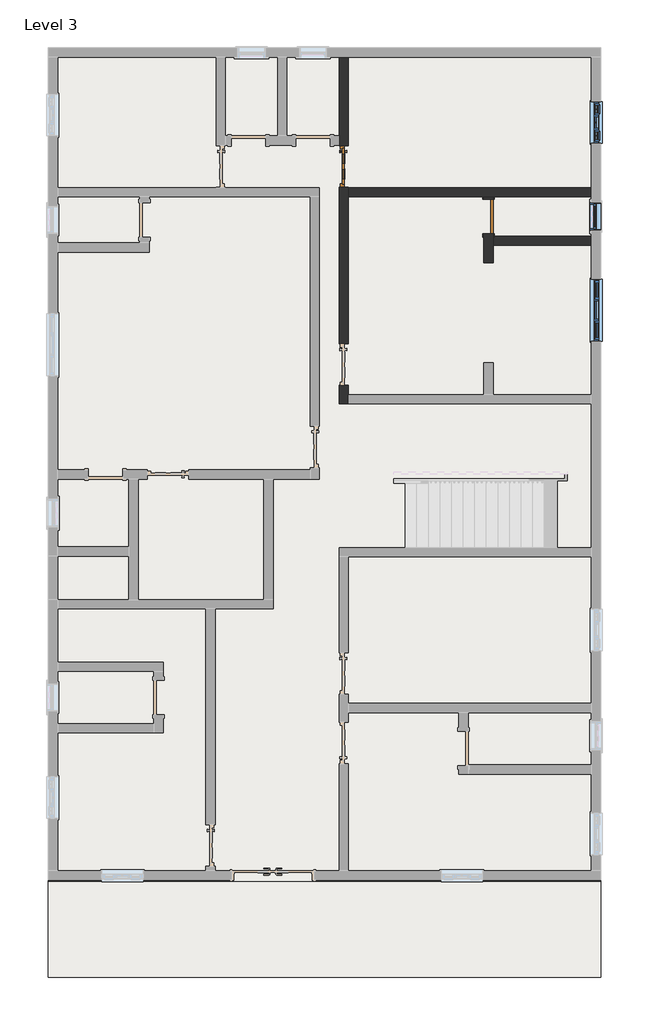
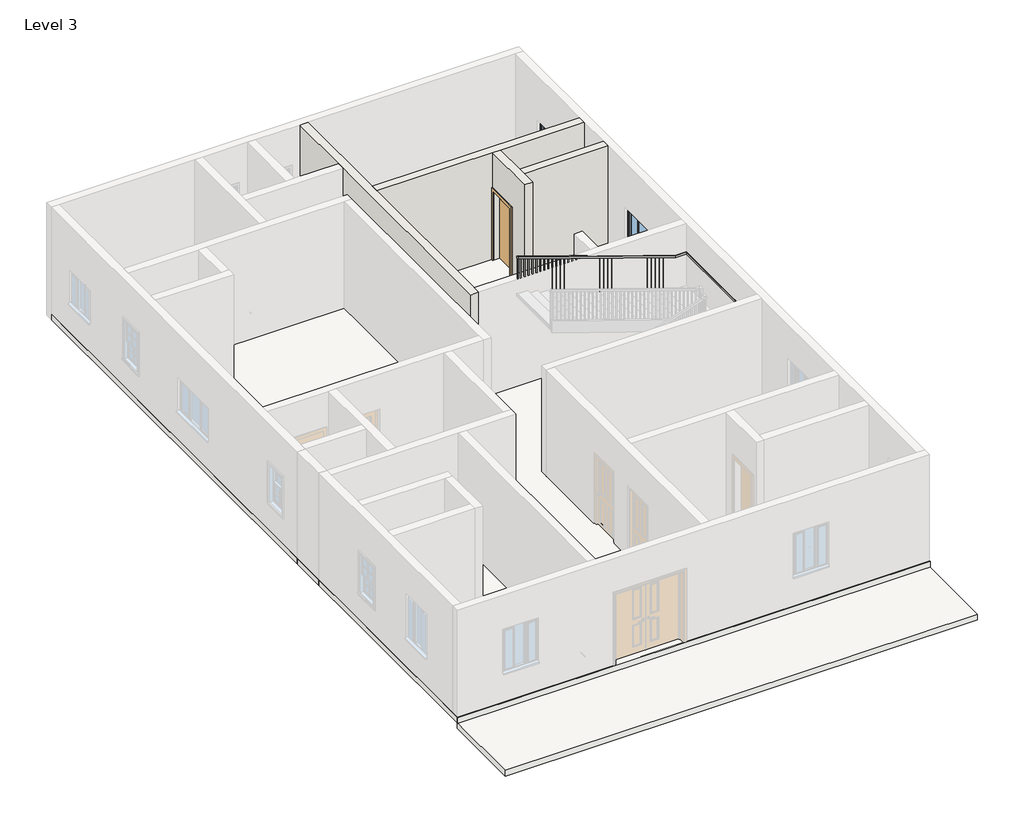
# One storey, part 2 of 3: 4 walls, 3 roofs, 3 windows, 2 doors, 1 railing, 1 slab.
"""IFC4 building model written with IfcOpenShell, lengths in millimetres."""

from ifc_helpers import new_model, si_unit, frame, origin, place, context, project, spatial, polyline, outline, extrude, faceted_brep, transform, mapped, element, save
from components import door_51b0c682, door_fadea3f2, window_679d2811, windows_tpl_plain_1360x910mm_84993ef1, windows_tpl_w_glazing_cross_bars_910x910mm_4aa0f884

model = new_model("IFC4")

# Units and contexts
model_context = context("Model", 3, world=origin())
ifc_project = project(units=[si_unit("LENGTHUNIT", "METRE", prefix="MILLI")], contexts=[model_context])

# Site, building, storey
site = spatial("IfcSite", under=ifc_project)
building = spatial("IfcBuilding", under=site)
storey = spatial("IfcBuildingStorey", under=building, Name="Level 3", Elevation=6096.0)

# Doors
placement = place(None, origin())
door_shape = door_51b0c682(model_context)
element("IfcDoor", 1, ObjectType="Doors_ExtSgl_2 : 2'x7\"", at=placement, inside=storey, context=model_context, shape_type="MappedRepresentation", body=[
    mapped(door_shape, transform((348.5548051, 6357.8803322, 6096.0), x_axis=(0.0, -1.0, 0.0), y_axis=(1.0, 0.0, 0.0), z_axis=(0.0, 0.0, 1.0))),
])
door_2_shape = door_fadea3f2(model_context)
element("IfcDoor", 2, ObjectType="Single-Flush : 30\" x 80\"", at=placement, inside=storey, context=model_context, shape_type="MappedRepresentation", body=[
    mapped(door_2_shape, transform((3523.5548051, 5259.3303322, 6096.0), x_axis=(0.0, -1.0, 0.0), y_axis=(1.0, 0.0, 0.0), z_axis=(0.0, 0.0, 1.0))),
])

# Railing
element("IfcRailing", 3, ObjectType="Handrail - Rectangular", at=placement, inside=storey, context=model_context, shape_type="SolidModel", body=[
    faceted_brep([(1449.3932247, -2014.4659014, 7096.125), (1449.3932247, -2014.4659014, 7042.4913852), (1449.3932247, -2065.2659014, 7042.4913852), (1449.3932247, -2065.2659014, 7096.125), (5246.6669505, -2014.4659014, 8382.0), (5255.0348019, -2014.4659014, 8331.2), (5255.0348019, -2065.2659014, 8331.2), (5246.6669505, -2065.2659014, 8382.0), (5771.4548051, -2014.4659014, 8382.0), (5771.4548051, -2014.4659014, 8331.2), (5822.2548051, -2065.2659014, 8331.2), (5822.2548051, -2065.2659014, 8382.0), (5771.4548051, 1135.1340986, 8382.0), (5771.4548051, 1135.1340986, 8331.2), (5822.2548051, 1185.9340986, 8331.2), (5822.2548051, 1185.9340986, 8382.0), (5499.8185322, 1135.1340986, 8382.0), (5491.4506807, 1135.1340986, 8331.2), (5491.4506807, 1185.9340986, 8331.2), (5499.8185322, 1185.9340986, 8382.0), (1449.3932247, 1135.1340986, 9753.6), (1449.3932247, 1185.9340986, 9753.6), (1449.3932247, 1185.9340986, 9699.9663852), (1449.3932247, 1135.1340986, 9699.9663852)], [[[0, 1, 2, 3]], [[1, 0, 4, 5]], [[2, 1, 5, 6]], [[3, 2, 6, 7]], [[0, 3, 7, 4]], [[5, 4, 8, 9]], [[6, 5, 9, 10]], [[7, 6, 10, 11]], [[4, 7, 11, 8]], [[9, 8, 12, 13]], [[10, 9, 13, 14]], [[11, 10, 14, 15]], [[8, 11, 15, 12]], [[13, 12, 16, 17]], [[14, 13, 17, 18]], [[15, 14, 18, 19]], [[12, 15, 19, 16]], [[20, 21, 22, 23]], [[17, 16, 20, 23]], [[18, 17, 23, 22]], [[19, 18, 22, 21]], [[16, 19, 21, 20]]]),
    extrude(outline(polyline([(9669.5618562, 1539.1798051), (9676.0127788, 1520.1298051), (8753.475, 1520.1298051), (8753.475, 1539.1798051), (9669.5618562, 1539.1798051)])), frame((0.0, 1151.0090986, 0.0), z_axis=(0.0, 1.0, 0.0), x_axis=(0.0, 0.0, 1.0)), (0.0, 0.0, 1.0), 19.05),
    extrude(outline(polyline([(9635.1569359, 1640.7798051), (9641.6078585, 1621.7298051), (8753.475, 1621.7298051), (8753.475, 1640.7798051), (9635.1569359, 1640.7798051)])), frame((0.0, 1151.0090986, 0.0), z_axis=(0.0, 1.0, 0.0), x_axis=(0.0, 0.0, 1.0)), (0.0, 0.0, 1.0), 19.05),
    extrude(outline(polyline([(9600.7520156, 1742.3798051), (9607.2029381, 1723.3298051), (8667.75, 1723.3298051), (8667.75, 1742.3798051), (9600.7520156, 1742.3798051)])), frame((0.0, 1151.0090986, 0.0), z_axis=(0.0, 1.0, 0.0), x_axis=(0.0, 0.0, 1.0)), (0.0, 0.0, 1.0), 19.05),
    extrude(outline(polyline([(9566.3470953, 1843.9798051), (9572.7980178, 1824.9298051), (8667.75, 1824.9298051), (8667.75, 1843.9798051), (9566.3470953, 1843.9798051)])), frame((0.0, 1151.0090986, 0.0), z_axis=(0.0, 1.0, 0.0), x_axis=(0.0, 0.0, 1.0)), (0.0, 0.0, 1.0), 19.05),
    extrude(outline(polyline([(9531.9421749, 1945.5798051), (9538.3930975, 1926.5298051), (8667.75, 1926.5298051), (8667.75, 1945.5798051), (9531.9421749, 1945.5798051)])), frame((0.0, 1151.0090986, 0.0), z_axis=(0.0, 1.0, 0.0), x_axis=(0.0, 0.0, 1.0)), (0.0, 0.0, 1.0), 19.05),
    extrude(outline(polyline([(9497.5372546, 2047.1798051), (9503.9881772, 2028.1298051), (8582.025, 2028.1298051), (8582.025, 2047.1798051), (9497.5372546, 2047.1798051)])), frame((0.0, 1151.0090986, 0.0), z_axis=(0.0, 1.0, 0.0), x_axis=(0.0, 0.0, 1.0)), (0.0, 0.0, 1.0), 19.05),
    extrude(outline(polyline([(9463.1323343, 2148.7798051), (9469.5832568, 2129.7298051), (8582.025, 2129.7298051), (8582.025, 2148.7798051), (9463.1323343, 2148.7798051)])), frame((0.0, 1151.0090986, 0.0), z_axis=(0.0, 1.0, 0.0), x_axis=(0.0, 0.0, 1.0)), (0.0, 0.0, 1.0), 19.05),
    extrude(outline(polyline([(9428.7274139, 2250.3798051), (9435.1783365, 2231.3298051), (8496.3, 2231.3298051), (8496.3, 2250.3798051), (9428.7274139, 2250.3798051)])), frame((0.0, 1151.0090986, 0.0), z_axis=(0.0, 1.0, 0.0), x_axis=(0.0, 0.0, 1.0)), (0.0, 0.0, 1.0), 19.05),
    extrude(outline(polyline([(9394.3224936, 2351.9798051), (9400.7734162, 2332.9298051), (8496.3, 2332.9298051), (8496.3, 2351.9798051), (9394.3224936, 2351.9798051)])), frame((0.0, 1151.0090986, 0.0), z_axis=(0.0, 1.0, 0.0), x_axis=(0.0, 0.0, 1.0)), (0.0, 0.0, 1.0), 19.05),
    extrude(outline(polyline([(9359.9175733, 2453.5798051), (9366.3684958, 2434.5298051), (8496.3, 2434.5298051), (8496.3, 2453.5798051), (9359.9175733, 2453.5798051)])), frame((0.0, 1151.0090986, 0.0), z_axis=(0.0, 1.0, 0.0), x_axis=(0.0, 0.0, 1.0)), (0.0, 0.0, 1.0), 19.05),
    extrude(outline(polyline([(9325.512653, 2555.1798051), (9331.9635755, 2536.1298051), (8410.575, 2536.1298051), (8410.575, 2555.1798051), (9325.512653, 2555.1798051)])), frame((0.0, 1151.0090986, 0.0), z_axis=(0.0, 1.0, 0.0), x_axis=(0.0, 0.0, 1.0)), (0.0, 0.0, 1.0), 19.05),
    extrude(outline(polyline([(9291.1077326, 2656.7798051), (9297.5586552, 2637.7298051), (8410.575, 2637.7298051), (8410.575, 2656.7798051), (9291.1077326, 2656.7798051)])), frame((0.0, 1151.0090986, 0.0), z_axis=(0.0, 1.0, 0.0), x_axis=(0.0, 0.0, 1.0)), (0.0, 0.0, 1.0), 19.05),
    extrude(outline(polyline([(9256.7028123, 2758.3798051), (9263.1537349, 2739.3298051), (8324.85, 2739.3298051), (8324.85, 2758.3798051), (9256.7028123, 2758.3798051)])), frame((0.0, 1151.0090986, 0.0), z_axis=(0.0, 1.0, 0.0), x_axis=(0.0, 0.0, 1.0)), (0.0, 0.0, 1.0), 19.05),
    extrude(outline(polyline([(9222.297892, 2859.9798051), (9228.7488145, 2840.9298051), (8324.85, 2840.9298051), (8324.85, 2859.9798051), (9222.297892, 2859.9798051)])), frame((0.0, 1151.0090986, 0.0), z_axis=(0.0, 1.0, 0.0), x_axis=(0.0, 0.0, 1.0)), (0.0, 0.0, 1.0), 19.05),
    extrude(outline(polyline([(9187.8929716, 2961.5798051), (9194.3438942, 2942.5298051), (8324.85, 2942.5298051), (8324.85, 2961.5798051), (9187.8929716, 2961.5798051)])), frame((0.0, 1151.0090986, 0.0), z_axis=(0.0, 1.0, 0.0), x_axis=(0.0, 0.0, 1.0)), (0.0, 0.0, 1.0), 19.05),
    extrude(outline(polyline([(9153.4880513, 3063.1798051), (9159.9389739, 3044.1298051), (8239.125, 3044.1298051), (8239.125, 3063.1798051), (9153.4880513, 3063.1798051)])), frame((0.0, 1151.0090986, 0.0), z_axis=(0.0, 1.0, 0.0), x_axis=(0.0, 0.0, 1.0)), (0.0, 0.0, 1.0), 19.05),
    extrude(outline(polyline([(9119.083131, 3164.7798051), (9125.5340535, 3145.7298051), (8239.125, 3145.7298051), (8239.125, 3164.7798051), (9119.083131, 3164.7798051)])), frame((0.0, 1151.0090986, 0.0), z_axis=(0.0, 1.0, 0.0), x_axis=(0.0, 0.0, 1.0)), (0.0, 0.0, 1.0), 19.05),
    extrude(outline(polyline([(9084.6782106, 3266.3798051), (9091.1291332, 3247.3298051), (8153.4, 3247.3298051), (8153.4, 3266.3798051), (9084.6782106, 3266.3798051)])), frame((0.0, 1151.0090986, 0.0), z_axis=(0.0, 1.0, 0.0), x_axis=(0.0, 0.0, 1.0)), (0.0, 0.0, 1.0), 19.05),
    extrude(outline(polyline([(9050.2732903, 3367.9798051), (9056.7242129, 3348.9298051), (8153.4, 3348.9298051), (8153.4, 3367.9798051), (9050.2732903, 3367.9798051)])), frame((0.0, 1151.0090986, 0.0), z_axis=(0.0, 1.0, 0.0), x_axis=(0.0, 0.0, 1.0)), (0.0, 0.0, 1.0), 19.05),
    extrude(outline(polyline([(9015.86837, 3469.5798051), (9022.3192926, 3450.5298051), (8153.4, 3450.5298051), (8153.4, 3469.5798051), (9015.86837, 3469.5798051)])), frame((0.0, 1151.0090986, 0.0), z_axis=(0.0, 1.0, 0.0), x_axis=(0.0, 0.0, 1.0)), (0.0, 0.0, 1.0), 19.05),
    extrude(outline(polyline([(8981.4634497, 3571.1798051), (8987.9143722, 3552.1298051), (8067.675, 3552.1298051), (8067.675, 3571.1798051), (8981.4634497, 3571.1798051)])), frame((0.0, 1151.0090986, 0.0), z_axis=(0.0, 1.0, 0.0), x_axis=(0.0, 0.0, 1.0)), (0.0, 0.0, 1.0), 19.05),
    extrude(outline(polyline([(8947.0585293, 3672.7798051), (8953.5094519, 3653.7298051), (8067.675, 3653.7298051), (8067.675, 3672.7798051), (8947.0585293, 3672.7798051)])), frame((0.0, 1151.0090986, 0.0), z_axis=(0.0, 1.0, 0.0), x_axis=(0.0, 0.0, 1.0)), (0.0, 0.0, 1.0), 19.05),
    extrude(outline(polyline([(8912.653609, 3774.3798051), (8919.1045316, 3755.3298051), (7981.95, 3755.3298051), (7981.95, 3774.3798051), (8912.653609, 3774.3798051)])), frame((0.0, 1151.0090986, 0.0), z_axis=(0.0, 1.0, 0.0), x_axis=(0.0, 0.0, 1.0)), (0.0, 0.0, 1.0), 19.05),
    extrude(outline(polyline([(8878.2486887, 3875.9798051), (8884.6996112, 3856.9298051), (7981.95, 3856.9298051), (7981.95, 3875.9798051), (8878.2486887, 3875.9798051)])), frame((0.0, 1151.0090986, 0.0), z_axis=(0.0, 1.0, 0.0), x_axis=(0.0, 0.0, 1.0)), (0.0, 0.0, 1.0), 19.05),
    extrude(outline(polyline([(8843.8437683, 3977.5798051), (8850.2946909, 3958.5298051), (7981.95, 3958.5298051), (7981.95, 3977.5798051), (8843.8437683, 3977.5798051)])), frame((0.0, 1151.0090986, 0.0), z_axis=(0.0, 1.0, 0.0), x_axis=(0.0, 0.0, 1.0)), (0.0, 0.0, 1.0), 19.05),
    extrude(outline(polyline([(8809.438848, 4079.1798051), (8815.8897706, 4060.1298051), (7896.225, 4060.1298051), (7896.225, 4079.1798051), (8809.438848, 4079.1798051)])), frame((0.0, 1151.0090986, 0.0), z_axis=(0.0, 1.0, 0.0), x_axis=(0.0, 0.0, 1.0)), (0.0, 0.0, 1.0), 19.05),
    extrude(outline(polyline([(8775.0339277, 4180.7798051), (8781.4848502, 4161.7298051), (7896.225, 4161.7298051), (7896.225, 4180.7798051), (8775.0339277, 4180.7798051)])), frame((0.0, 1151.0090986, 0.0), z_axis=(0.0, 1.0, 0.0), x_axis=(0.0, 0.0, 1.0)), (0.0, 0.0, 1.0), 19.05),
    extrude(outline(polyline([(8740.6290074, 4282.3798051), (8747.0799299, 4263.3298051), (7810.5, 4263.3298051), (7810.5, 4282.3798051), (8740.6290074, 4282.3798051)])), frame((0.0, 1151.0090986, 0.0), z_axis=(0.0, 1.0, 0.0), x_axis=(0.0, 0.0, 1.0)), (0.0, 0.0, 1.0), 19.05),
    extrude(outline(polyline([(8706.224087, 4383.9798051), (8712.6750096, 4364.9298051), (7810.5, 4364.9298051), (7810.5, 4383.9798051), (8706.224087, 4383.9798051)])), frame((0.0, 1151.0090986, 0.0), z_axis=(0.0, 1.0, 0.0), x_axis=(0.0, 0.0, 1.0)), (0.0, 0.0, 1.0), 19.05),
    extrude(outline(polyline([(8671.8191667, 4485.5798051), (8678.2700893, 4466.5298051), (7810.5, 4466.5298051), (7810.5, 4485.5798051), (8671.8191667, 4485.5798051)])), frame((0.0, 1151.0090986, 0.0), z_axis=(0.0, 1.0, 0.0), x_axis=(0.0, 0.0, 1.0)), (0.0, 0.0, 1.0), 19.05),
    extrude(outline(polyline([(8637.4142464, 4587.1798051), (8643.8651689, 4568.1298051), (7724.775, 4568.1298051), (7724.775, 4587.1798051), (8637.4142464, 4587.1798051)])), frame((0.0, 1151.0090986, 0.0), z_axis=(0.0, 1.0, 0.0), x_axis=(0.0, 0.0, 1.0)), (0.0, 0.0, 1.0), 19.05),
    extrude(outline(polyline([(8603.009326, 4688.7798051), (8609.4602486, 4669.7298051), (7724.775, 4669.7298051), (7724.775, 4688.7798051), (8603.009326, 4688.7798051)])), frame((0.0, 1151.0090986, 0.0), z_axis=(0.0, 1.0, 0.0), x_axis=(0.0, 0.0, 1.0)), (0.0, 0.0, 1.0), 19.05),
    extrude(outline(polyline([(8568.6044057, 4790.3798051), (8575.0553283, 4771.3298051), (7639.05, 4771.3298051), (7639.05, 4790.3798051), (8568.6044057, 4790.3798051)])), frame((0.0, 1151.0090986, 0.0), z_axis=(0.0, 1.0, 0.0), x_axis=(0.0, 0.0, 1.0)), (0.0, 0.0, 1.0), 19.05),
    extrude(outline(polyline([(8534.1994854, 4891.9798051), (8540.6504079, 4872.9298051), (7639.05, 4872.9298051), (7639.05, 4891.9798051), (8534.1994854, 4891.9798051)])), frame((0.0, 1151.0090986, 0.0), z_axis=(0.0, 1.0, 0.0), x_axis=(0.0, 0.0, 1.0)), (0.0, 0.0, 1.0), 19.05),
    extrude(outline(polyline([(8499.8163852, 4993.5798051), (8506.2673078, 4974.5298051), (7639.05, 4974.5298051), (7639.05, 4993.5798051), (8499.8163852, 4993.5798051)])), frame((0.0, 1151.0090986, 0.0), z_axis=(0.0, 1.0, 0.0), x_axis=(0.0, 0.0, 1.0)), (0.0, 0.0, 1.0), 19.05),
    extrude(outline(polyline([(8465.3896447, 5095.1798051), (8471.8405673, 5076.1298051), (7553.325, 5076.1298051), (7553.325, 5095.1798051), (8465.3896447, 5095.1798051)])), frame((0.0, 1151.0090986, 0.0), z_axis=(0.0, 1.0, 0.0), x_axis=(0.0, 0.0, 1.0)), (0.0, 0.0, 1.0), 19.05),
    extrude(outline(polyline([(8430.9847244, 5196.7798051), (8437.435647, 5177.7298051), (7553.325, 5177.7298051), (7553.325, 5196.7798051), (8430.9847244, 5196.7798051)])), frame((0.0, 1151.0090986, 0.0), z_axis=(0.0, 1.0, 0.0), x_axis=(0.0, 0.0, 1.0)), (0.0, 0.0, 1.0), 19.05),
    extrude(outline(polyline([(8396.5798041, 5298.3798051), (8403.0307266, 5279.3298051), (7467.6, 5279.3298051), (7467.6, 5298.3798051), (8396.5798041, 5298.3798051)])), frame((0.0, 1151.0090986, 0.0), z_axis=(0.0, 1.0, 0.0), x_axis=(0.0, 0.0, 1.0)), (0.0, 0.0, 1.0), 19.05),
    extrude(outline(polyline([(8362.1748837, 5399.9798051), (8368.6258063, 5380.9298051), (7467.6, 5380.9298051), (7467.6, 5399.9798051), (8362.1748837, 5399.9798051)])), frame((0.0, 1151.0090986, 0.0), z_axis=(0.0, 1.0, 0.0), x_axis=(0.0, 0.0, 1.0)), (0.0, 0.0, 1.0), 19.05),
    extrude(outline(polyline([(8327.7699634, 5501.5798051), (8334.220886, 5482.5298051), (7467.6, 5482.5298051), (7467.6, 5501.5798051), (8327.7699634, 5501.5798051)])), frame((0.0, 1151.0090986, 0.0), z_axis=(0.0, 1.0, 0.0), x_axis=(0.0, 0.0, 1.0)), (0.0, 0.0, 1.0), 19.05),
    extrude(outline(polyline([(5603.1798051, 1170.0590986), (5603.1798051, 1151.0090986), (5584.1298051, 1151.0090986), (5584.1298051, 1170.0590986), (5603.1798051, 1170.0590986)])), frame((0.0, 0.0, 7467.6), z_axis=(0.0, 0.0, 1.0), x_axis=(1.0, 0.0, 0.0)), (0.0, 0.0, 1.0), 863.6),
    extrude(outline(polyline([(5704.7798051, 1170.0590986), (5704.7798051, 1151.0090986), (5685.7298051, 1151.0090986), (5685.7298051, 1170.0590986), (5704.7798051, 1170.0590986)])), frame((0.0, 0.0, 7467.6), z_axis=(0.0, 0.0, 1.0), x_axis=(1.0, 0.0, 0.0)), (0.0, 0.0, 1.0), 863.6),
    extrude(outline(polyline([(5806.3798051, 1100.2090986), (5787.3298051, 1100.2090986), (5787.3298051, 1119.2590986), (5806.3798051, 1119.2590986), (5806.3798051, 1100.2090986)])), frame((0.0, 0.0, 7467.6), z_axis=(0.0, 0.0, 1.0), x_axis=(1.0, 0.0, 0.0)), (0.0, 0.0, 1.0), 863.6),
    extrude(outline(polyline([(5806.3798051, 998.6090986), (5787.3298051, 998.6090986), (5787.3298051, 1017.6590986), (5806.3798051, 1017.6590986), (5806.3798051, 998.6090986)])), frame((0.0, 0.0, 7467.6), z_axis=(0.0, 0.0, 1.0), x_axis=(1.0, 0.0, 0.0)), (0.0, 0.0, 1.0), 863.6),
    extrude(outline(polyline([(5806.3798051, 897.0090986), (5787.3298051, 897.0090986), (5787.3298051, 916.0590986), (5806.3798051, 916.0590986), (5806.3798051, 897.0090986)])), frame((0.0, 0.0, 7467.6), z_axis=(0.0, 0.0, 1.0), x_axis=(1.0, 0.0, 0.0)), (0.0, 0.0, 1.0), 863.6),
    extrude(outline(polyline([(5806.3798051, 795.4090986), (5787.3298051, 795.4090986), (5787.3298051, 814.4590986), (5806.3798051, 814.4590986), (5806.3798051, 795.4090986)])), frame((0.0, 0.0, 7467.6), z_axis=(0.0, 0.0, 1.0), x_axis=(1.0, 0.0, 0.0)), (0.0, 0.0, 1.0), 863.6),
    extrude(outline(polyline([(5806.3798051, 693.8090986), (5787.3298051, 693.8090986), (5787.3298051, 712.8590986), (5806.3798051, 712.8590986), (5806.3798051, 693.8090986)])), frame((0.0, 0.0, 7467.6), z_axis=(0.0, 0.0, 1.0), x_axis=(1.0, 0.0, 0.0)), (0.0, 0.0, 1.0), 863.6),
    extrude(outline(polyline([(5806.3798051, 592.2090986), (5787.3298051, 592.2090986), (5787.3298051, 611.2590986), (5806.3798051, 611.2590986), (5806.3798051, 592.2090986)])), frame((0.0, 0.0, 7467.6), z_axis=(0.0, 0.0, 1.0), x_axis=(1.0, 0.0, 0.0)), (0.0, 0.0, 1.0), 863.6),
    extrude(outline(polyline([(5806.3798051, 490.6090986), (5787.3298051, 490.6090986), (5787.3298051, 509.6590986), (5806.3798051, 509.6590986), (5806.3798051, 490.6090986)])), frame((0.0, 0.0, 7467.6), z_axis=(0.0, 0.0, 1.0), x_axis=(1.0, 0.0, 0.0)), (0.0, 0.0, 1.0), 863.6),
    extrude(outline(polyline([(5806.3798051, 389.0090986), (5787.3298051, 389.0090986), (5787.3298051, 408.0590986), (5806.3798051, 408.0590986), (5806.3798051, 389.0090986)])), frame((0.0, 0.0, 7467.6), z_axis=(0.0, 0.0, 1.0), x_axis=(1.0, 0.0, 0.0)), (0.0, 0.0, 1.0), 863.6),
    extrude(outline(polyline([(5806.3798051, 287.4090986), (5787.3298051, 287.4090986), (5787.3298051, 306.4590986), (5806.3798051, 306.4590986), (5806.3798051, 287.4090986)])), frame((0.0, 0.0, 7467.6), z_axis=(0.0, 0.0, 1.0), x_axis=(1.0, 0.0, 0.0)), (0.0, 0.0, 1.0), 863.6),
    extrude(outline(polyline([(5806.3798051, 185.8090986), (5787.3298051, 185.8090986), (5787.3298051, 204.8590986), (5806.3798051, 204.8590986), (5806.3798051, 185.8090986)])), frame((0.0, 0.0, 7467.6), z_axis=(0.0, 0.0, 1.0), x_axis=(1.0, 0.0, 0.0)), (0.0, 0.0, 1.0), 863.6),
    extrude(outline(polyline([(5806.3798051, 84.2090986), (5787.3298051, 84.2090986), (5787.3298051, 103.2590986), (5806.3798051, 103.2590986), (5806.3798051, 84.2090986)])), frame((0.0, 0.0, 7467.6), z_axis=(0.0, 0.0, 1.0), x_axis=(1.0, 0.0, 0.0)), (0.0, 0.0, 1.0), 863.6),
    extrude(outline(polyline([(5806.3798051, -17.3909014), (5787.3298051, -17.3909014), (5787.3298051, 1.6590986), (5806.3798051, 1.6590986), (5806.3798051, -17.3909014)])), frame((0.0, 0.0, 7467.6), z_axis=(0.0, 0.0, 1.0), x_axis=(1.0, 0.0, 0.0)), (0.0, 0.0, 1.0), 863.6),
    extrude(outline(polyline([(5806.3798051, -118.9909014), (5787.3298051, -118.9909014), (5787.3298051, -99.9409014), (5806.3798051, -99.9409014), (5806.3798051, -118.9909014)])), frame((0.0, 0.0, 7467.6), z_axis=(0.0, 0.0, 1.0), x_axis=(1.0, 0.0, 0.0)), (0.0, 0.0, 1.0), 863.6),
    extrude(outline(polyline([(5806.3798051, -220.5909014), (5787.3298051, -220.5909014), (5787.3298051, -201.5409014), (5806.3798051, -201.5409014), (5806.3798051, -220.5909014)])), frame((0.0, 0.0, 7467.6), z_axis=(0.0, 0.0, 1.0), x_axis=(1.0, 0.0, 0.0)), (0.0, 0.0, 1.0), 863.6),
    extrude(outline(polyline([(5806.3798051, -322.1909014), (5787.3298051, -322.1909014), (5787.3298051, -303.1409014), (5806.3798051, -303.1409014), (5806.3798051, -322.1909014)])), frame((0.0, 0.0, 7467.6), z_axis=(0.0, 0.0, 1.0), x_axis=(1.0, 0.0, 0.0)), (0.0, 0.0, 1.0), 863.6),
    extrude(outline(polyline([(5806.3798051, -423.7909014), (5787.3298051, -423.7909014), (5787.3298051, -404.7409014), (5806.3798051, -404.7409014), (5806.3798051, -423.7909014)])), frame((0.0, 0.0, 7467.6), z_axis=(0.0, 0.0, 1.0), x_axis=(1.0, 0.0, 0.0)), (0.0, 0.0, 1.0), 863.6),
    extrude(outline(polyline([(5806.3798051, -525.3909014), (5787.3298051, -525.3909014), (5787.3298051, -506.3409014), (5806.3798051, -506.3409014), (5806.3798051, -525.3909014)])), frame((0.0, 0.0, 7467.6), z_axis=(0.0, 0.0, 1.0), x_axis=(1.0, 0.0, 0.0)), (0.0, 0.0, 1.0), 863.6),
    extrude(outline(polyline([(5806.3798051, -626.9909014), (5787.3298051, -626.9909014), (5787.3298051, -607.9409014), (5806.3798051, -607.9409014), (5806.3798051, -626.9909014)])), frame((0.0, 0.0, 7467.6), z_axis=(0.0, 0.0, 1.0), x_axis=(1.0, 0.0, 0.0)), (0.0, 0.0, 1.0), 863.6),
    extrude(outline(polyline([(5806.3798051, -728.5909014), (5787.3298051, -728.5909014), (5787.3298051, -709.5409014), (5806.3798051, -709.5409014), (5806.3798051, -728.5909014)])), frame((0.0, 0.0, 7467.6), z_axis=(0.0, 0.0, 1.0), x_axis=(1.0, 0.0, 0.0)), (0.0, 0.0, 1.0), 863.6),
    extrude(outline(polyline([(5806.3798051, -830.1909014), (5787.3298051, -830.1909014), (5787.3298051, -811.1409014), (5806.3798051, -811.1409014), (5806.3798051, -830.1909014)])), frame((0.0, 0.0, 7467.6), z_axis=(0.0, 0.0, 1.0), x_axis=(1.0, 0.0, 0.0)), (0.0, 0.0, 1.0), 863.6),
    extrude(outline(polyline([(5806.3798051, -931.7909014), (5787.3298051, -931.7909014), (5787.3298051, -912.7409014), (5806.3798051, -912.7409014), (5806.3798051, -931.7909014)])), frame((0.0, 0.0, 7467.6), z_axis=(0.0, 0.0, 1.0), x_axis=(1.0, 0.0, 0.0)), (0.0, 0.0, 1.0), 863.6),
    extrude(outline(polyline([(5806.3798051, -1033.3909014), (5787.3298051, -1033.3909014), (5787.3298051, -1014.3409014), (5806.3798051, -1014.3409014), (5806.3798051, -1033.3909014)])), frame((0.0, 0.0, 7467.6), z_axis=(0.0, 0.0, 1.0), x_axis=(1.0, 0.0, 0.0)), (0.0, 0.0, 1.0), 863.6),
    extrude(outline(polyline([(5806.3798051, -1134.9909014), (5787.3298051, -1134.9909014), (5787.3298051, -1115.9409014), (5806.3798051, -1115.9409014), (5806.3798051, -1134.9909014)])), frame((0.0, 0.0, 7467.6), z_axis=(0.0, 0.0, 1.0), x_axis=(1.0, 0.0, 0.0)), (0.0, 0.0, 1.0), 863.6),
    extrude(outline(polyline([(5806.3798051, -1236.5909014), (5787.3298051, -1236.5909014), (5787.3298051, -1217.5409014), (5806.3798051, -1217.5409014), (5806.3798051, -1236.5909014)])), frame((0.0, 0.0, 7467.6), z_axis=(0.0, 0.0, 1.0), x_axis=(1.0, 0.0, 0.0)), (0.0, 0.0, 1.0), 863.6),
    extrude(outline(polyline([(5806.3798051, -1338.1909014), (5787.3298051, -1338.1909014), (5787.3298051, -1319.1409014), (5806.3798051, -1319.1409014), (5806.3798051, -1338.1909014)])), frame((0.0, 0.0, 7467.6), z_axis=(0.0, 0.0, 1.0), x_axis=(1.0, 0.0, 0.0)), (0.0, 0.0, 1.0), 863.6),
    extrude(outline(polyline([(5806.3798051, -1439.7909014), (5787.3298051, -1439.7909014), (5787.3298051, -1420.7409014), (5806.3798051, -1420.7409014), (5806.3798051, -1439.7909014)])), frame((0.0, 0.0, 7467.6), z_axis=(0.0, 0.0, 1.0), x_axis=(1.0, 0.0, 0.0)), (0.0, 0.0, 1.0), 863.6),
    extrude(outline(polyline([(5806.3798051, -1541.3909014), (5787.3298051, -1541.3909014), (5787.3298051, -1522.3409014), (5806.3798051, -1522.3409014), (5806.3798051, -1541.3909014)])), frame((0.0, 0.0, 7467.6), z_axis=(0.0, 0.0, 1.0), x_axis=(1.0, 0.0, 0.0)), (0.0, 0.0, 1.0), 863.6),
    extrude(outline(polyline([(5806.3798051, -1642.9909014), (5787.3298051, -1642.9909014), (5787.3298051, -1623.9409014), (5806.3798051, -1623.9409014), (5806.3798051, -1642.9909014)])), frame((0.0, 0.0, 7467.6), z_axis=(0.0, 0.0, 1.0), x_axis=(1.0, 0.0, 0.0)), (0.0, 0.0, 1.0), 863.6),
    extrude(outline(polyline([(5806.3798051, -1744.5909014), (5787.3298051, -1744.5909014), (5787.3298051, -1725.5409014), (5806.3798051, -1725.5409014), (5806.3798051, -1744.5909014)])), frame((0.0, 0.0, 7467.6), z_axis=(0.0, 0.0, 1.0), x_axis=(1.0, 0.0, 0.0)), (0.0, 0.0, 1.0), 863.6),
    extrude(outline(polyline([(5806.3798051, -1846.1909014), (5787.3298051, -1846.1909014), (5787.3298051, -1827.1409014), (5806.3798051, -1827.1409014), (5806.3798051, -1846.1909014)])), frame((0.0, 0.0, 7467.6), z_axis=(0.0, 0.0, 1.0), x_axis=(1.0, 0.0, 0.0)), (0.0, 0.0, 1.0), 863.6),
    extrude(outline(polyline([(5806.3798051, -1947.7909014), (5787.3298051, -1947.7909014), (5787.3298051, -1928.7409014), (5806.3798051, -1928.7409014), (5806.3798051, -1947.7909014)])), frame((0.0, 0.0, 7467.6), z_axis=(0.0, 0.0, 1.0), x_axis=(1.0, 0.0, 0.0)), (0.0, 0.0, 1.0), 863.6),
    extrude(outline(polyline([(5707.0682247, -2049.3909014), (5707.0682247, -2030.3409014), (5726.1182247, -2030.3409014), (5726.1182247, -2049.3909014), (5707.0682247, -2049.3909014)])), frame((0.0, 0.0, 7467.6), z_axis=(0.0, 0.0, 1.0), x_axis=(1.0, 0.0, 0.0)), (0.0, 0.0, 1.0), 863.6),
    extrude(outline(polyline([(5605.4682247, -2049.3909014), (5605.4682247, -2030.3409014), (5624.5182247, -2030.3409014), (5624.5182247, -2049.3909014), (5605.4682247, -2049.3909014)])), frame((0.0, 0.0, 7467.6), z_axis=(0.0, 0.0, 1.0), x_axis=(1.0, 0.0, 0.0)), (0.0, 0.0, 1.0), 863.6),
    extrude(outline(polyline([(5503.8682247, -2049.3909014), (5503.8682247, -2030.3409014), (5522.9182247, -2030.3409014), (5522.9182247, -2049.3909014), (5503.8682247, -2049.3909014)])), frame((0.0, 0.0, 7467.6), z_axis=(0.0, 0.0, 1.0), x_axis=(1.0, 0.0, 0.0)), (0.0, 0.0, 1.0), 863.6),
    extrude(outline(polyline([(5402.2682247, -2049.3909014), (5402.2682247, -2030.3409014), (5421.3182247, -2030.3409014), (5421.3182247, -2049.3909014), (5402.2682247, -2049.3909014)])), frame((0.0, 0.0, 7467.6), z_axis=(0.0, 0.0, 1.0), x_axis=(1.0, 0.0, 0.0)), (0.0, 0.0, 1.0), 863.6),
    extrude(outline(polyline([(5300.6682247, -2049.3909014), (5300.6682247, -2030.3409014), (5319.7182247, -2030.3409014), (5319.7182247, -2049.3909014), (5300.6682247, -2049.3909014)])), frame((0.0, 0.0, 7467.6), z_axis=(0.0, 0.0, 1.0), x_axis=(1.0, 0.0, 0.0)), (0.0, 0.0, 1.0), 863.6),
    extrude(outline(polyline([(8318.6988987, 5218.1182247), (8312.2479761, 5199.0682247), (7381.875, 5199.0682247), (7381.875, 5218.1182247), (8318.6988987, 5218.1182247)])), frame((0.0, -2049.3909014, 0.0), z_axis=(0.0, 1.0, 0.0), x_axis=(0.0, 0.0, 1.0)), (0.0, 0.0, 1.0), 19.05),
    extrude(outline(polyline([(8284.2939783, 5116.5182247), (8277.8430558, 5097.4682247), (7381.875, 5097.4682247), (7381.875, 5116.5182247), (8284.2939783, 5116.5182247)])), frame((0.0, -2049.3909014, 0.0), z_axis=(0.0, 1.0, 0.0), x_axis=(0.0, 0.0, 1.0)), (0.0, 0.0, 1.0), 19.05),
    extrude(outline(polyline([(8249.889058, 5014.9182247), (8243.4381354, 4995.8682247), (7381.875, 4995.8682247), (7381.875, 5014.9182247), (8249.889058, 5014.9182247)])), frame((0.0, -2049.3909014, 0.0), z_axis=(0.0, 1.0, 0.0), x_axis=(0.0, 0.0, 1.0)), (0.0, 0.0, 1.0), 19.05),
    extrude(outline(polyline([(8215.4841377, 4913.3182247), (8209.0332151, 4894.2682247), (7296.15, 4894.2682247), (7296.15, 4913.3182247), (8215.4841377, 4913.3182247)])), frame((0.0, -2049.3909014, 0.0), z_axis=(0.0, 1.0, 0.0), x_axis=(0.0, 0.0, 1.0)), (0.0, 0.0, 1.0), 19.05),
    extrude(outline(polyline([(8181.0792173, 4811.7182247), (8174.6282948, 4792.6682247), (7296.15, 4792.6682247), (7296.15, 4811.7182247), (8181.0792173, 4811.7182247)])), frame((0.0, -2049.3909014, 0.0), z_axis=(0.0, 1.0, 0.0), x_axis=(0.0, 0.0, 1.0)), (0.0, 0.0, 1.0), 19.05),
    extrude(outline(polyline([(8146.674297, 4710.1182247), (8140.2233745, 4691.0682247), (7210.425, 4691.0682247), (7210.425, 4710.1182247), (8146.674297, 4710.1182247)])), frame((0.0, -2049.3909014, 0.0), z_axis=(0.0, 1.0, 0.0), x_axis=(0.0, 0.0, 1.0)), (0.0, 0.0, 1.0), 19.05),
    extrude(outline(polyline([(8112.2693767, 4608.5182247), (8105.8184541, 4589.4682247), (7210.425, 4589.4682247), (7210.425, 4608.5182247), (8112.2693767, 4608.5182247)])), frame((0.0, -2049.3909014, 0.0), z_axis=(0.0, 1.0, 0.0), x_axis=(0.0, 0.0, 1.0)), (0.0, 0.0, 1.0), 19.05),
    extrude(outline(polyline([(8077.8644564, 4506.9182247), (8071.4135338, 4487.8682247), (7210.425, 4487.8682247), (7210.425, 4506.9182247), (8077.8644564, 4506.9182247)])), frame((0.0, -2049.3909014, 0.0), z_axis=(0.0, 1.0, 0.0), x_axis=(0.0, 0.0, 1.0)), (0.0, 0.0, 1.0), 19.05),
    extrude(outline(polyline([(8043.459536, 4405.3182247), (8037.0086135, 4386.2682247), (7124.7, 4386.2682247), (7124.7, 4405.3182247), (8043.459536, 4405.3182247)])), frame((0.0, -2049.3909014, 0.0), z_axis=(0.0, 1.0, 0.0), x_axis=(0.0, 0.0, 1.0)), (0.0, 0.0, 1.0), 19.05),
    extrude(outline(polyline([(8009.0546157, 4303.7182247), (8002.6036931, 4284.6682247), (7124.7, 4284.6682247), (7124.7, 4303.7182247), (8009.0546157, 4303.7182247)])), frame((0.0, -2049.3909014, 0.0), z_axis=(0.0, 1.0, 0.0), x_axis=(0.0, 0.0, 1.0)), (0.0, 0.0, 1.0), 19.05),
    extrude(outline(polyline([(7974.6496954, 4202.1182247), (7968.1987728, 4183.0682247), (7038.975, 4183.0682247), (7038.975, 4202.1182247), (7974.6496954, 4202.1182247)])), frame((0.0, -2049.3909014, 0.0), z_axis=(0.0, 1.0, 0.0), x_axis=(0.0, 0.0, 1.0)), (0.0, 0.0, 1.0), 19.05),
    extrude(outline(polyline([(7940.244775, 4100.5182247), (7933.7938525, 4081.4682247), (7038.975, 4081.4682247), (7038.975, 4100.5182247), (7940.244775, 4100.5182247)])), frame((0.0, -2049.3909014, 0.0), z_axis=(0.0, 1.0, 0.0), x_axis=(0.0, 0.0, 1.0)), (0.0, 0.0, 1.0), 19.05),
    extrude(outline(polyline([(7905.8398547, 3998.9182247), (7899.3889321, 3979.8682247), (7038.975, 3979.8682247), (7038.975, 3998.9182247), (7905.8398547, 3998.9182247)])), frame((0.0, -2049.3909014, 0.0), z_axis=(0.0, 1.0, 0.0), x_axis=(0.0, 0.0, 1.0)), (0.0, 0.0, 1.0), 19.05),
    extrude(outline(polyline([(7871.4349344, 3897.3182247), (7864.9840118, 3878.2682247), (6953.25, 3878.2682247), (6953.25, 3897.3182247), (7871.4349344, 3897.3182247)])), frame((0.0, -2049.3909014, 0.0), z_axis=(0.0, 1.0, 0.0), x_axis=(0.0, 0.0, 1.0)), (0.0, 0.0, 1.0), 19.05),
    extrude(outline(polyline([(7837.0300141, 3795.7182247), (7830.5790915, 3776.6682247), (6953.25, 3776.6682247), (6953.25, 3795.7182247), (7837.0300141, 3795.7182247)])), frame((0.0, -2049.3909014, 0.0), z_axis=(0.0, 1.0, 0.0), x_axis=(0.0, 0.0, 1.0)), (0.0, 0.0, 1.0), 19.05),
    extrude(outline(polyline([(7802.6250937, 3694.1182247), (7796.1741712, 3675.0682247), (6867.525, 3675.0682247), (6867.525, 3694.1182247), (7802.6250937, 3694.1182247)])), frame((0.0, -2049.3909014, 0.0), z_axis=(0.0, 1.0, 0.0), x_axis=(0.0, 0.0, 1.0)), (0.0, 0.0, 1.0), 19.05),
    extrude(outline(polyline([(7768.2201734, 3592.5182247), (7761.7692508, 3573.4682247), (6867.525, 3573.4682247), (6867.525, 3592.5182247), (7768.2201734, 3592.5182247)])), frame((0.0, -2049.3909014, 0.0), z_axis=(0.0, 1.0, 0.0), x_axis=(0.0, 0.0, 1.0)), (0.0, 0.0, 1.0), 19.05),
    extrude(outline(polyline([(7733.8152531, 3490.9182247), (7727.3643305, 3471.8682247), (6867.525, 3471.8682247), (6867.525, 3490.9182247), (7733.8152531, 3490.9182247)])), frame((0.0, -2049.3909014, 0.0), z_axis=(0.0, 1.0, 0.0), x_axis=(0.0, 0.0, 1.0)), (0.0, 0.0, 1.0), 19.05),
    extrude(outline(polyline([(7699.4103327, 3389.3182247), (7692.9594102, 3370.2682247), (6781.8, 3370.2682247), (6781.8, 3389.3182247), (7699.4103327, 3389.3182247)])), frame((0.0, -2049.3909014, 0.0), z_axis=(0.0, 1.0, 0.0), x_axis=(0.0, 0.0, 1.0)), (0.0, 0.0, 1.0), 19.05),
    extrude(outline(polyline([(7665.0054124, 3287.7182247), (7658.5544898, 3268.6682247), (6781.8, 3268.6682247), (6781.8, 3287.7182247), (7665.0054124, 3287.7182247)])), frame((0.0, -2049.3909014, 0.0), z_axis=(0.0, 1.0, 0.0), x_axis=(0.0, 0.0, 1.0)), (0.0, 0.0, 1.0), 19.05),
    extrude(outline(polyline([(7630.6004921, 3186.1182247), (7624.1495695, 3167.0682247), (6696.075, 3167.0682247), (6696.075, 3186.1182247), (7630.6004921, 3186.1182247)])), frame((0.0, -2049.3909014, 0.0), z_axis=(0.0, 1.0, 0.0), x_axis=(0.0, 0.0, 1.0)), (0.0, 0.0, 1.0), 19.05),
    extrude(outline(polyline([(7596.1955718, 3084.5182247), (7589.7446492, 3065.4682247), (6696.075, 3065.4682247), (6696.075, 3084.5182247), (7596.1955718, 3084.5182247)])), frame((0.0, -2049.3909014, 0.0), z_axis=(0.0, 1.0, 0.0), x_axis=(0.0, 0.0, 1.0)), (0.0, 0.0, 1.0), 19.05),
    extrude(outline(polyline([(7561.7906514, 2982.9182247), (7555.3397289, 2963.8682247), (6696.075, 2963.8682247), (6696.075, 2982.9182247), (7561.7906514, 2982.9182247)])), frame((0.0, -2049.3909014, 0.0), z_axis=(0.0, 1.0, 0.0), x_axis=(0.0, 0.0, 1.0)), (0.0, 0.0, 1.0), 19.05),
    extrude(outline(polyline([(7527.3857311, 2881.3182247), (7520.9348085, 2862.2682247), (6610.35, 2862.2682247), (6610.35, 2881.3182247), (7527.3857311, 2881.3182247)])), frame((0.0, -2049.3909014, 0.0), z_axis=(0.0, 1.0, 0.0), x_axis=(0.0, 0.0, 1.0)), (0.0, 0.0, 1.0), 19.05),
    extrude(outline(polyline([(7492.9808108, 2779.7182247), (7486.5298882, 2760.6682247), (6610.35, 2760.6682247), (6610.35, 2779.7182247), (7492.9808108, 2779.7182247)])), frame((0.0, -2049.3909014, 0.0), z_axis=(0.0, 1.0, 0.0), x_axis=(0.0, 0.0, 1.0)), (0.0, 0.0, 1.0), 19.05),
    extrude(outline(polyline([(7458.5758904, 2678.1182247), (7452.1249679, 2659.0682247), (6524.625, 2659.0682247), (6524.625, 2678.1182247), (7458.5758904, 2678.1182247)])), frame((0.0, -2049.3909014, 0.0), z_axis=(0.0, 1.0, 0.0), x_axis=(0.0, 0.0, 1.0)), (0.0, 0.0, 1.0), 19.05),
    extrude(outline(polyline([(7424.1709701, 2576.5182247), (7417.7200475, 2557.4682247), (6524.625, 2557.4682247), (6524.625, 2576.5182247), (7424.1709701, 2576.5182247)])), frame((0.0, -2049.3909014, 0.0), z_axis=(0.0, 1.0, 0.0), x_axis=(0.0, 0.0, 1.0)), (0.0, 0.0, 1.0), 19.05),
    extrude(outline(polyline([(7389.7660498, 2474.9182247), (7383.3151272, 2455.8682247), (6524.625, 2455.8682247), (6524.625, 2474.9182247), (7389.7660498, 2474.9182247)])), frame((0.0, -2049.3909014, 0.0), z_axis=(0.0, 1.0, 0.0), x_axis=(0.0, 0.0, 1.0)), (0.0, 0.0, 1.0), 19.05),
    extrude(outline(polyline([(7355.3611294, 2373.3182247), (7348.9102069, 2354.2682247), (6438.9, 2354.2682247), (6438.9, 2373.3182247), (7355.3611294, 2373.3182247)])), frame((0.0, -2049.3909014, 0.0), z_axis=(0.0, 1.0, 0.0), x_axis=(0.0, 0.0, 1.0)), (0.0, 0.0, 1.0), 19.05),
    extrude(outline(polyline([(7320.9562091, 2271.7182247), (7314.5052866, 2252.6682247), (6438.9, 2252.6682247), (6438.9, 2271.7182247), (7320.9562091, 2271.7182247)])), frame((0.0, -2049.3909014, 0.0), z_axis=(0.0, 1.0, 0.0), x_axis=(0.0, 0.0, 1.0)), (0.0, 0.0, 1.0), 19.05),
    extrude(outline(polyline([(7286.5512888, 2170.1182247), (7280.1003662, 2151.0682247), (6353.175, 2151.0682247), (6353.175, 2170.1182247), (7286.5512888, 2170.1182247)])), frame((0.0, -2049.3909014, 0.0), z_axis=(0.0, 1.0, 0.0), x_axis=(0.0, 0.0, 1.0)), (0.0, 0.0, 1.0), 19.05),
    extrude(outline(polyline([(7252.1463685, 2068.5182247), (7245.6954459, 2049.4682247), (6353.175, 2049.4682247), (6353.175, 2068.5182247), (7252.1463685, 2068.5182247)])), frame((0.0, -2049.3909014, 0.0), z_axis=(0.0, 1.0, 0.0), x_axis=(0.0, 0.0, 1.0)), (0.0, 0.0, 1.0), 19.05),
    extrude(outline(polyline([(7217.7414481, 1966.9182247), (7211.2905256, 1947.8682247), (6353.175, 1947.8682247), (6353.175, 1966.9182247), (7217.7414481, 1966.9182247)])), frame((0.0, -2049.3909014, 0.0), z_axis=(0.0, 1.0, 0.0), x_axis=(0.0, 0.0, 1.0)), (0.0, 0.0, 1.0), 19.05),
    extrude(outline(polyline([(7183.3365278, 1865.3182247), (7176.8856052, 1846.2682247), (6267.45, 1846.2682247), (6267.45, 1865.3182247), (7183.3365278, 1865.3182247)])), frame((0.0, -2049.3909014, 0.0), z_axis=(0.0, 1.0, 0.0), x_axis=(0.0, 0.0, 1.0)), (0.0, 0.0, 1.0), 19.05),
    extrude(outline(polyline([(7148.9316075, 1763.7182247), (7142.4806849, 1744.6682247), (6267.45, 1744.6682247), (6267.45, 1763.7182247), (7148.9316075, 1763.7182247)])), frame((0.0, -2049.3909014, 0.0), z_axis=(0.0, 1.0, 0.0), x_axis=(0.0, 0.0, 1.0)), (0.0, 0.0, 1.0), 19.05),
    extrude(outline(polyline([(7114.5266871, 1662.1182247), (7108.0757646, 1643.0682247), (6181.725, 1643.0682247), (6181.725, 1662.1182247), (7114.5266871, 1662.1182247)])), frame((0.0, -2049.3909014, 0.0), z_axis=(0.0, 1.0, 0.0), x_axis=(0.0, 0.0, 1.0)), (0.0, 0.0, 1.0), 19.05),
    extrude(outline(polyline([(7080.1217668, 1560.5182247), (7073.6708443, 1541.4682247), (6181.725, 1541.4682247), (6181.725, 1560.5182247), (7080.1217668, 1560.5182247)])), frame((0.0, -2049.3909014, 0.0), z_axis=(0.0, 1.0, 0.0), x_axis=(0.0, 0.0, 1.0)), (0.0, 0.0, 1.0), 19.05),
    extrude(outline(polyline([(5806.3798051, 1151.0090986), (5787.3298051, 1151.0090986), (5787.3298051, 1170.0590986), (5806.3798051, 1170.0590986), (5806.3798051, 1151.0090986)])), frame((0.0, 0.0, 7467.6), z_axis=(0.0, 0.0, 1.0), x_axis=(1.0, 0.0, 0.0)), (0.0, 0.0, 1.0), 863.6),
    extrude(outline(polyline([(5787.3298051, -2049.3909014), (5787.3298051, -2030.3409014), (5806.3798051, -2030.3409014), (5806.3798051, -2049.3909014), (5787.3298051, -2049.3909014)])), frame((0.0, 0.0, 7467.6), z_axis=(0.0, 0.0, 1.0), x_axis=(1.0, 0.0, 0.0)), (0.0, 0.0, 1.0), 863.6),
    extrude(outline(polyline([(9693.5154626, 1468.4432247), (9699.9663852, 1449.3932247), (8753.475, 1449.3932247), (8753.475, 1468.4432247), (9693.5154626, 1468.4432247)])), frame((0.0, 1151.0090986, 0.0), z_axis=(0.0, 1.0, 0.0), x_axis=(0.0, 0.0, 1.0)), (0.0, 0.0, 1.0), 19.05),
    extrude(outline(polyline([(7048.9423078, 1468.4432247), (7042.4913852, 1449.3932247), (6181.725, 1449.3932247), (6181.725, 1468.4432247), (7048.9423078, 1468.4432247)])), frame((0.0, -2049.3909014, 0.0), z_axis=(0.0, 1.0, 0.0), x_axis=(0.0, 0.0, 1.0)), (0.0, 0.0, 1.0), 19.05),
])

# Roofs
element("IfcRoof", 4, ObjectType="Generic - 12\"", at=placement, inside=storey, context=model_context, shape_type="SweptSolid", body=[
    extrude(outline(polyline([(-6134.0560205, 8955.7974079), (5981.7439795, 8955.7974079), (5981.7439795, -9323.5734342), (-6134.0560205, -9323.5734342), (-6134.0560205, 8955.7974079)])), frame((0.0, 0.0, 6096.0), z_axis=(0.0, 0.0, 1.0), x_axis=(1.0, 0.0, 0.0)), (0.0, 0.0, 1.0), 152.4),
])
element("IfcRoof", 5, ObjectType="Generic - 12\"", at=placement, inside=storey, context=model_context, shape_type="SweptSolid", body=[
    extrude(outline(polyline([(-6134.0560205, 8955.7974079), (5981.7439795, 8955.7974079), (5981.7439795, -9298.1734342), (-6134.0560205, -9298.1734342), (-6134.0560205, 8955.7974079)])), frame((0.0, 0.0, 6096.0), z_axis=(0.0, 0.0, 1.0), x_axis=(1.0, 0.0, 0.0)), (0.0, 0.0, 1.0), 152.4),
])
element("IfcRoof", 6, ObjectType="Generic - 12\"", at=placement, inside=storey, context=model_context, shape_type="SweptSolid", body=[
    extrude(outline(polyline([(-6134.0560205, 8955.7974079), (5981.7439795, 8955.7974079), (5981.7439795, -9323.5734342), (-6134.0560205, -9323.5734342), (-6134.0560205, 8955.7974079)])), frame((0.0, 0.0, 6096.0), z_axis=(0.0, 0.0, 1.0), x_axis=(1.0, 0.0, 0.0)), (0.0, 0.0, 1.0), 152.4),
])

# Slab
element("IfcSlab", 7, ObjectType="Generic - 12\"", at=placement, inside=storey, context=model_context, shape_type="SweptSolid", body=[
    extrude(outline(polyline([(5981.7439795, -9298.1734342), (5981.7439795, -11431.7734342), (-6134.0560205, -11431.7734342), (-6134.0560205, -9298.1734342), (5981.7439795, -9298.1734342)])), frame((0.0, 0.0, 5943.6), z_axis=(0.0, 0.0, 1.0), x_axis=(1.0, 0.0, 0.0)), (0.0, 0.0, 1.0), 152.4),
])

# Walls
element("IfcWall", 8, ObjectType="Generic - 4.5\" p", at=placement, inside=storey, context=model_context, shape_type="Brep", body=[
    faceted_brep([(246.9548051, 1556.4340986, 8206.0), (246.9548051, 1556.4340986, 6096.0), (246.9548051, 1147.8340986, 6096.0), (246.9548051, 1147.8340986, 9144.0), (246.9548051, 6824.7340986, 9144.0), (246.9548051, 7027.9340986, 9144.0), (246.9548051, 8752.5974079, 9144.0), (246.9548051, 8752.5974079, 6096.0), (246.9548051, 7027.9340986, 6096.0), (246.9548051, 6824.7340986, 6096.0), (246.9548051, 6812.8803322, 6096.0), (246.9548051, 6812.8803322, 8206.0), (246.9548051, 5902.8803322, 8206.0), (246.9548051, 5902.8803322, 6096.0), (246.9548051, 2466.4340986, 6096.0), (246.9548051, 2466.4340986, 8206.0), (450.1548051, 1147.8340986, 6096.0), (450.1548051, 1351.0340986, 6096.0), (450.1548051, 1556.4340986, 6096.0), (450.1548051, 1556.4340986, 8206.0), (450.1548051, 2466.4340986, 8206.0), (450.1548051, 2466.4340986, 6096.0), (450.1548051, 5687.8265658, 6096.0), (450.1548051, 5891.0265658, 6096.0), (450.1548051, 5902.8803322, 6096.0), (450.1548051, 5902.8803322, 8206.0), (450.1548051, 6812.8803322, 8206.0), (450.1548051, 6812.8803322, 6096.0), (450.1548051, 8752.5974079, 6096.0), (450.1548051, 8752.5974079, 9144.0), (450.1548051, 5891.0265658, 9144.0), (450.1548051, 5687.8265658, 9144.0), (450.1548051, 1351.0340986, 9144.0), (450.1548051, 1147.8340986, 9144.0)], [[[0, 1, 2, 3, 4, 5, 6, 7, 8, 9, 10, 11, 12, 13, 14, 15]], [[16, 17, 18, 19, 20, 21, 22, 23, 24, 25, 26, 27, 28, 29, 30, 31, 32, 33]], [[10, 9, 8, 7, 28, 27]], [[14, 13, 24, 23, 22, 21]], [[2, 1, 18, 17, 16]], [[7, 6, 29, 28]], [[3, 2, 16, 33]], [[27, 26, 11, 10]], [[25, 24, 13, 12]], [[26, 25, 12, 11]], [[21, 20, 15, 14]], [[19, 18, 1, 0]], [[20, 19, 0, 15]], [[6, 5, 4, 3, 33, 32, 31, 30, 29]]]),
])
element("IfcWall", 9, ObjectType="Generic - 4.5\" p", at=placement, inside=storey, context=model_context, shape_type="Brep", body=[
    faceted_brep([(450.1548051, 5687.8265658, 6096.0), (3421.9548051, 5687.8265658, 6096.0), (3625.1548051, 5687.8265658, 6096.0), (5778.5439795, 5687.8265658, 6096.0), (5778.5439795, 5687.8265658, 9144.0), (3625.1548051, 5687.8265658, 9144.0), (3421.9548051, 5687.8265658, 9144.0), (450.1548051, 5687.8265658, 9144.0), (450.1548051, 5891.0265658, 6096.0), (450.1548051, 5891.0265658, 9144.0), (5778.5439795, 5891.0265658, 9144.0), (5778.5439795, 5891.0265658, 6096.0)], [[[0, 1, 2, 3, 4, 5, 6, 7]], [[8, 9, 10, 11]], [[3, 2, 1, 0, 8, 11]], [[4, 3, 11, 10]], [[0, 7, 9, 8]], [[7, 6, 5, 4, 10, 9]]]),
])
element("IfcWall", 10, ObjectType="Generic - 4.5\" p", at=placement, inside=storey, context=model_context, shape_type="Brep", body=[
    faceted_brep([(3421.9548051, 4878.3303322, 8128.0), (3421.9548051, 4878.3303322, 6096.0), (3421.9548051, 4247.7840898, 6096.0), (3421.9548051, 4247.7840898, 9144.0), (3421.9548051, 5687.8265658, 9144.0), (3421.9548051, 5687.8265658, 6096.0), (3421.9548051, 5640.3303322, 6096.0), (3421.9548051, 5640.3303322, 8128.0), (3625.1548051, 4247.7840898, 6096.0), (3625.1548051, 4627.6340986, 6096.0), (3625.1548051, 4830.8340986, 6096.0), (3625.1548051, 4878.3303322, 6096.0), (3625.1548051, 4878.3303322, 8128.0), (3625.1548051, 5640.3303322, 8128.0), (3625.1548051, 5640.3303322, 6096.0), (3625.1548051, 5687.8265658, 6096.0), (3625.1548051, 5687.8265658, 9144.0), (3625.1548051, 4830.8340986, 9144.0), (3625.1548051, 4627.6340986, 9144.0), (3625.1548051, 4247.7840898, 9144.0)], [[[0, 1, 2, 3, 4, 5, 6, 7]], [[8, 9, 10, 11, 12, 13, 14, 15, 16, 17, 18, 19]], [[6, 5, 15, 14]], [[2, 1, 11, 10, 9, 8]], [[3, 2, 8, 19]], [[5, 4, 16, 15]], [[12, 11, 1, 0]], [[13, 12, 0, 7]], [[14, 13, 7, 6]], [[4, 3, 19, 18, 17, 16]]]),
])
element("IfcWall", 11, ObjectType="Generic - 4.5\" p", at=placement, inside=storey, context=model_context, shape_type="SweptSolid", body=[
    extrude(outline(polyline([(5778.5439795, 4627.6340986), (3625.1548051, 4627.6340986), (3625.1548051, 4830.8340986), (5778.5439795, 4830.8340986), (5778.5439795, 4627.6340986)])), frame((0.0, 0.0, 6096.0), z_axis=(0.0, 0.0, 1.0), x_axis=(1.0, 0.0, 0.0)), (0.0, 0.0, 1.0), 3048.0),
])

# Windows
window_shape = window_679d2811(model_context)
element("IfcWindow", 12, ObjectType="Window-Double-Hung : 24\" x 42\"", at=placement, inside=storey, context=model_context, shape_type="MappedRepresentation", body=[
    mapped(window_shape, transform((5880.1439795, 5259.3303322, 6096.0), x_axis=(0.0, 1.0, 0.0), y_axis=(-1.0, 0.0, 0.0), z_axis=(0.0, 0.0, 1.0))),
])
windows_tpl_plain_1360x910mm_shape = windows_tpl_plain_1360x910mm_84993ef1(model_context)
element("IfcWindow", 13, ObjectType="Windows_Tpl_Plain : 1360x910mm", at=placement, inside=storey, context=model_context, shape_type="MappedRepresentation", body=[
    mapped(windows_tpl_plain_1360x910mm_shape, transform((5871.6874117, 2703.567432, 5810.4), x_axis=(0.0, -1.0, 0.0), y_axis=(1.0, 0.0, 0.0), z_axis=(0.0, 0.0, 1.0))),
])
windows_tpl_w_glazing_cross_bars_910x910mm_shape = windows_tpl_w_glazing_cross_bars_910x910mm_4aa0f884(model_context)
element("IfcWindow", 14, ObjectType="Windows_Tpl_w-Glazing_Cross-Bars : 910x910mm", at=placement, inside=storey, context=model_context, shape_type="MappedRepresentation", body=[
    mapped(windows_tpl_w_glazing_cross_bars_910x910mm_shape, transform((5871.6874117, 6895.1453202, 5810.4), x_axis=(0.0, -1.0, 0.0), y_axis=(1.0, 0.0, 0.0), z_axis=(0.0, 0.0, 1.0))),
])

save(model, "model.ifc")

# Revit data of these elements
# Type "Doors_ExtSgl_2 : 2'x7\""
#   Type Mark = "10"
#   Type Comments = "External Single"
#   Operation = "SingleSwingRight"
#   Construction Type Id = "SGL"
#   Keynote = "L20"
#   Analytic Construction = "Large single-glazed windows"
#   Wrap Layers (Int) from Ext = 0' - 6.98819"
#   Wrap Layers (Ext) from Ext = 0' - 4.03543"
#   Visual Light Transmittance = 0.9
#   Thickness = 0' - 1.73228"
#   Stile Top of Lock rail = 3' - 3.37008"
#   Stile Top Rail = 0' - 5.90551"
#   Stile Shutting = 0' - 4.92126"
#   Stile Muntin Rail = 0' - 4.92126"
#   Stile Lock Rail = 0' - 6.88976"
#   Stile Hanging = 0' - 4.92126"
#   Stile Bottom Rail = 0' - 6.88976"
#   Solar Heat Gain Coefficient = 0.86
#   Rough Width = 2' - 11.82677"
#   Rough Height = 6' - 11.07087"
#   O/A Frame Width = 0' - 2.51969"
#   Heat Transfer Coefficient (U) = 0.979472 BTU/(h·ft²·°F)
#   Handle Z Distance = 3' - 3.37008"
#   Glazing Thickness = 0' - 0.94488"
#   FrameWidth = 0' - 1.65354"
#   FrameOffset - External = 0' - 0.98425"
#   FrameDepth = 0' - 3.50394"
#   Door Panel Width = 2' - 7.77165"
#   Door Panel Thickness = 0' - 1.73228"
#   Door Panel Height = 6' - 6.74016"
#   Cill Thickness = 0' - 2.14567"
#   Cill Projection = 0' - 1.1811"
#   Handle X Distance = 0' - 2.95276"
#   Height = 6' - 11.07087"
#   Structural Tolerance = 0' - 0.25591"
#   Tolerance = 0' - 0.11811"
#   Undercut = 0' - 0.15748"
#   Width = 2' - 11.82677"
#   Cill Extension = 0' - 0.98425"
#   Cavity Closer Width = 0' - 1.9685"
#   Cavity Closer Offset from Ext = 0' - 4.03543"
#   Cavity Closer Depth = 0' - 3.34646"
#   Vis - Ironmongery = yes
#   Vis - Cavity Closers = yes
#   Define Thermal Properties by = 1
#   Function = 1
#   Material Glass = Door - Glazing
#   Material Door = Door - Panel
#   Material Frame = Door - Frame/Mullion
#   Material Ironmongery = Door - Handle
#   Wall Closure = (empty or 0)
# Type "Single-Flush : 30\" x 80\""
#   Type Mark = "5"
#   Construction Type Id = "MDOOR"
#   Assembly Code = "C1020"
#   Analytic Construction = "Metal"
#   Thickness = 0' - 2"
#   Heat Transfer Coefficient (U) = 0.651978 BTU/(h·ft²·°F)
#   Height = 6' - 8"
#   Trim Projection Ext = 0' - 1"
#   Trim Projection Int = 0' - 1"
#   Trim Width = 0' - 3"
#   Width = 2' - 6"
#   Define Thermal Properties by = 1
#   Define Thermal Properties by = 1
#   Door Material = Door - Panel
#   Frame Material = Door - Frame
#   Visual Light Transmittance = 0
#   Solar Heat Gain Coefficient = 0
#   Function = (empty or 0)
#   Wall Closure = (empty or 0)
# Type "Handrail - Rectangular"
#   Assembly Code = "C2010400"
#   built-in parameter 1008612 = 0.0416667 (stored number, unit not read)
#   built-in parameter 1008611 = 0.0416667 (stored number, unit not read)
#   built-in parameter 1008609 = 0.333333 (stored number, unit not read)
#   built-in parameter 1008604 = 0.166667 (stored number, unit not read)
#   built-in parameter 1008603 = 0.166667 (stored number, unit not read)
#   Railing Height = 3' - 0"
#   built-in parameter 1008630 = 2
#   built-in parameter 1008610 = 2
#   built-in parameter 1008618 = Baluster - Square : 3/4"
# Type "Generic - 12\""
#   Assembly Code = "B1020"
#   Layers, outside or top first: 0' - 6" no material (function 1)
# Type "Generic - 12\""
#   Assembly Code = "B1010"
#   Function = 0
#   Layers, outside or top first: 0' - 6" no material (function 1)
# Type "Generic - 4.5\" p"
#   Assembly Code = "B2010"
#   Layers, outside or top first: 0' - 8" no material (function 1)
# Type "Window-Double-Hung : 24\" x 42\""
#   Type Mark = "10"
#   Fire Rating = "0.5h"
#   Construction Type Id = "DG-DR"
#   Assembly Code = "B2020100"
#   Analytic Construction = "Double glazing - domestic"
#   Wall Thickness [instance default] = 0' - 6"
#   Window Inset [instance default] = 0' - 0"
#   Visual Light Transmittance = 0.81
#   Thermal Resistance (R) = 1.8146 (h·ft²·°F)/BTU
#   Solar Heat Gain Coefficient = 0.76
#   Muntin Width = 1' - 6"
#   Muntin Height = 1' - 5 1/8"
#   Interior Wall Closure [instance default] = 0' - 1 1/2"
#   Rough Width = 2' - 0 1/2"
#   Rough Height = 3' - 6 1/2"
#   Frame Extension [instance default] = 0' - 1 1/4"
#   Exterior Wall Closure [instance default] = 0' - 0 1/2"
#   Extension Jamb [instance default] = 0' - 1 1/2"
#   Heat Transfer Coefficient (U) = 0.5511 BTU/(h·ft²·°F)
#   Height = 3' - 6"
#   Width = 2' - 0"
#   Define Thermal Properties by = 1
#   Top Muntin Visibility = yes
#   Indicator Visibility [instance default] = yes
#   Extension Jamb Visibility [instance default] = yes
#   Interior Trim Visibility [instance default] = yes
#   Exterior Trim Visibility [instance default] = yes
#   Define Thermal Properties by = 1
#   Bottom Muntin Visibility = yes
#   Muntin Pattern = Muntin Pattern_2x2 : Muntin Pattern_2x2
#   Interior Trim Material = Wood - Stained
#   Interior Trim = Trim-Window-Interior-Flat : Picture Frame
#   Exterior Trim Material = Clad - White
#   Exterior Trim = Trim-Window-Exterior-Flat : with Sill
#   Glass Panel Material = Glass
#   Exterior Frame Material = Clad - White
#   Interior Frame Material = Wood - Stained
#   Wall Closure = (empty or 0)
# Type "Windows_Tpl_Plain : 1360x910mm"
#   Type Mark = "20"
#   Operation = "TriplePanelVertical"
#   Construction Type Id = "GSP4R"
#   Manufacturer = "Revit"
#   Keynote = "L10"
#   Analytic Construction = "1/8 in Pilkington single glazing"
#   Wrap Layers (Ext) from Ext = 0' - 4.03543"
#   Wrap Layers (Int) from Ext = 0' - 6.98819"
#   Window Board Projection = 0' - 0.98425"
#   Window Board Extension = 0' - 0.98425"
#   Visual Light Transmittance = 0.9
#   Solar Heat Gain Coefficient = 0.78
#   Rough Width = 4' - 5.54331"
#   Rough Height = 2' - 11.82677"
#   Height = 2' - 11.82677"
#   Width = 4' - 5.54331"
#   Heat Transfer Coefficient (U) = 0.6496 BTU/(h·ft²·°F)
#   Glazing Thickness = 0' - 0.94488"
#   FrameOffset - External = 0' - 1.9685"
#   Frame Depth = 0' - 2.55906"
#   Default Head Height = 6' - 11.07087"
#   Cill Depth = 0' - 3.44488"
#   Cavity Closer Width = 0' - 1.9685"
#   Cavity Closer Offset from Ext = 0' - 4.03543"
#   Cavity Closer Depth = 0' - 3.34646"
#   Vis - Cavity Closers = yes
#   Define Thermal Properties by = 1
#   Material Trim = Window Frame
#   Material Glass = Glass
#   Material Frame = Window Frame
#   Wall Closure = (empty or 0)
# Type "Windows_Tpl_w-Glazing_Cross-Bars : 910x910mm"
#   Type Mark = "24"
#   Operation = "TriplePanelVertical"
#   Construction Type Id = "GSP4R"
#   Manufacturer = "Revit"
#   Keynote = "L10"
#   Analytic Construction = "1/8 in Pilkington single glazing"
#   Wrap Layers (Ext) from Ext = 0' - 4.03543"
